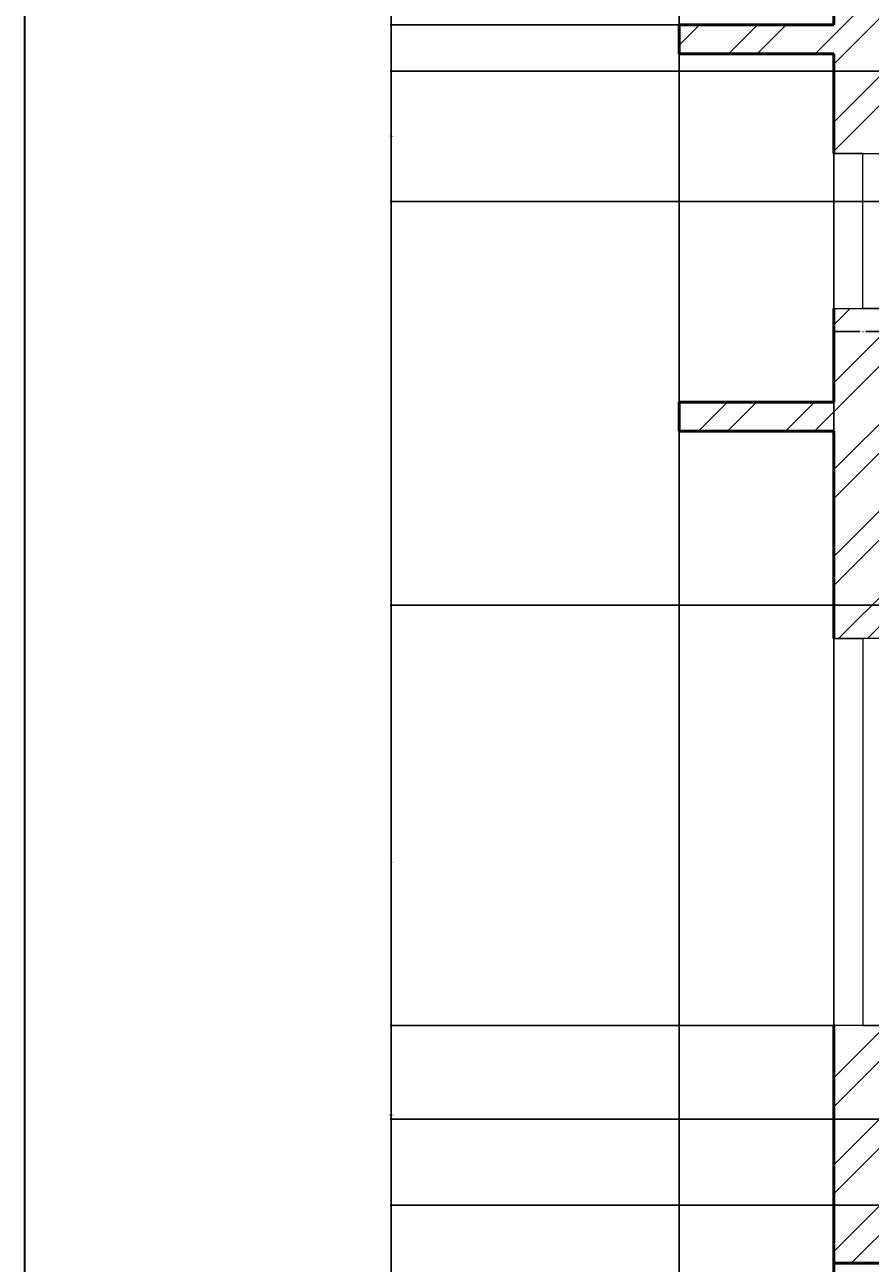
# Model space of a CAD drawing. Units: inches. Extents: x 1980 to 2738, y 1471 to 2568.
# Tile 2 of 22: x 1980 to 2111, y 1686 to 1878. Entities that reach past the tile are written whole.
import ezdxf

# ---------------------------------------------------------------- set-up
doc = ezdxf.new("R2010")
doc.units = ezdxf.units.IN
for name, color, linetype, lineweight in [('A-ANNO-DIMS', 2, 'Continuous', 18), ('A-ANNO-TTLB', 7, 'Continuous', 35), ('A-FLOR-BALC', 7, 'Continuous', 25), ('A-GLAZ', 141, 'Continuous', 18), ('A-WALL', 7, 'Continuous', 50)]:
    doc.layers.add(name, color=color, linetype=linetype, lineweight=lineweight)
doc.layers.add('A-WALL-PATT', color=9, linetype='Continuous', lineweight=13, true_color=0xd19cc7)
doc.styles.get("Standard").update_dxf_attribs({"font": 'arial.ttf'})
doc.dimstyles.get("Standard").update_dxf_attribs({"dimtxt": 0.18, "dimasz": 0.18, "dimexe": 0.18, "dimexo": 0.0625, "dimgap": 0.09, "dimtad": 0, "dimtih": 1, "dimtoh": 1, "dimdec": 4, "dimzin": 0, "dimdsep": 46, "dimtxsty": 'Standard', "dimcen": 0.09, "dimadec": 0, "dimazin": 0, "dimtfac": 1, "dimtdec": 4, "dimtofl": 0, "dimtmove": 0, "dimatfit": 3, "dimfxl": 1, "dimtolj": 1, "dimtzin": 0, "dimarcsym": 0})

# ---------------------------------------------------------------- blocks, each defined once
blk = doc.blocks.new('WIN-60IN-WALL')
for p, q in [((0, 9), (0, 0)), ((60, 9), (0, 9)), ((60, 4.5), (60, 9)), ((60, 9), (60, 0)), ((0, 0), (0, 4.5)), ((0, 4.5), (60, 4.5)), ((0, 0), (60, 0))]:
    blk.add_line(p, q)
blk = doc.blocks.new('WIN-24IN-WALL')
for p, q in [((4.5, 24), (0, 24)), ((0, 24), (9, 24)), ((0, 24), (0, 0)), ((4.5, 0), (4.5, 24)), ((9, 0), (9, 24)), ((0, 0), (9, 0)), ((9, 0), (4.5, 0))]:
    blk.add_line(p, q)
blk = doc.blocks.new('*D24')
at = {"layer": 'A-ANNO-DIMS', "color": 0, "lineweight": -2, "transparency": 16777216}
for p, q in [((2105.08, 1833.67), (2105.08, 1829.95)), ((2114.08, 1833.67), (2114.08, 1829.95)), ((2105.26, 1830.13), (2109.13, 1830.13)), ((2113.9, 1830.13), (2110.04, 1830.13))]:
    blk.add_line(p, q, dxfattribs=at)
at = {"layer": 'A-ANNO-DIMS', "color": 0, "transparency": 16777216}
for points in [[(2105.26, 1830.16), (2105.26, 1830.1), (2105.08, 1830.13)], [(2113.9, 1830.16), (2113.9, 1830.1), (2114.08, 1830.13)]]:
    blk.add_solid(points, dxfattribs=at)
at = {"layer": 'Defpoints', "color": 0, "transparency": 16777216}
for p in [(2105.08, 1833.73), (2114.08, 1833.73), (2114.08, 1830.13)]:
    blk.add_point(p, dxfattribs=at)
at = {"layer": 'A-ANNO-DIMS', "color": 0, "transparency": 16777216, "insert": (2109.58, 1830.13), "char_height": 0.18, "attachment_point": 5}
blk.add_mtext('\\A1;9 TYP.', dxfattribs=at)
blk = doc.blocks.new('*D36')
at = {"layer": 'A-ANNO-DIMS', "color": 0, "lineweight": -2, "transparency": 16777216}
for p, q in [((2105.02, 2462.71), (2036.25, 2462.71)), ((2036.43, 2462.53), (2036.43, 2053.39)), ((2036.43, 1643.89), (2036.43, 2053.02)), ((2105.02, 1643.71), (2036.25, 1643.71))]:
    blk.add_line(p, q, dxfattribs=at)
at = {"layer": 'A-ANNO-DIMS', "color": 0, "transparency": 16777216}
for points in [[(2036.4, 2462.53), (2036.46, 2462.53), (2036.43, 2462.71)], [(2036.4, 1643.89), (2036.46, 1643.89), (2036.43, 1643.71)]]:
    blk.add_solid(points, dxfattribs=at)
at = {"layer": 'Defpoints', "color": 0, "transparency": 16777216}
for p in [(2036.43, 2462.71), (2105.08, 2462.71), (2105.08, 1643.71)]:
    blk.add_point(p, dxfattribs=at)
at = {"layer": 'A-ANNO-DIMS', "color": 0, "transparency": 16777216, "insert": (2036.43, 2053.21), "char_height": 0.18, "attachment_point": 5}
blk.add_mtext('\\A1;819', dxfattribs=at)
blk = doc.blocks.new('*D48')
at = {"layer": 'A-ANNO-DIMS', "color": 0, "lineweight": -2, "transparency": 16777216}
for p, q in [((2081.08, 1873.14), (2081.08, 1533.71)), ((2105.08, 1873.14), (2105.08, 1533.71)), ((2081.26, 1533.89), (2092.86, 1533.89)), ((2104.9, 1533.89), (2093.3, 1533.89))]:
    blk.add_line(p, q, dxfattribs=at)
at = {"layer": 'A-ANNO-DIMS', "color": 0, "transparency": 16777216}
for points in [[(2081.26, 1533.92), (2081.26, 1533.86), (2081.08, 1533.89)], [(2104.9, 1533.92), (2104.9, 1533.86), (2105.08, 1533.89)]]:
    blk.add_solid(points, dxfattribs=at)
at = {"layer": 'Defpoints', "color": 0, "transparency": 16777216}
for p in [(2081.08, 1873.21), (2105.08, 1873.21), (2105.08, 1533.89)]:
    blk.add_point(p, dxfattribs=at)
at = {"layer": 'A-ANNO-DIMS', "color": 0, "transparency": 16777216, "insert": (2093.08, 1533.89), "char_height": 0.18, "attachment_point": 5}
blk.add_mtext('\\A1;24', dxfattribs=at)
blk = doc.blocks.new('*D49')
at = {"layer": 'A-ANNO-DIMS', "color": 0, "lineweight": -2, "transparency": 16777216}
for p, q in [((2105.02, 1722.55), (2036.25, 1722.55)), ((2036.43, 1722.37), (2036.43, 1708.81)), ((2036.43, 1694.89), (2036.43, 1708.45)), ((2114.02, 1694.71), (2036.25, 1694.71))]:
    blk.add_line(p, q, dxfattribs=at)
at = {"layer": 'A-ANNO-DIMS', "color": 0, "transparency": 16777216}
for points in [[(2036.4, 1722.37), (2036.46, 1722.37), (2036.43, 1722.55)], [(2036.4, 1694.89), (2036.46, 1694.89), (2036.43, 1694.71)]]:
    blk.add_solid(points, dxfattribs=at)
at = {"layer": 'Defpoints', "color": 0, "transparency": 16777216}
for p in [(2036.43, 1722.55), (2105.08, 1722.55), (2114.08, 1694.71)]:
    blk.add_point(p, dxfattribs=at)
at = {"layer": 'A-ANNO-DIMS', "color": 0, "transparency": 16777216, "insert": (2036.43, 1708.63), "char_height": 0.18, "attachment_point": 5}
blk.add_mtext('\\A1;27.845', dxfattribs=at)
blk = doc.blocks.new('*D52')
at = {"layer": 'A-ANNO-DIMS', "color": 0, "lineweight": -2, "transparency": 16777216}
for p, q in [((2341.71, 1787.71), (2036.25, 1787.71)), ((2036.43, 1787.53), (2036.43, 1748.05)), ((2036.43, 1708.21), (2036.43, 1747.69)), ((2341.71, 1708.03), (2036.25, 1708.03))]:
    blk.add_line(p, q, dxfattribs=at)
at = {"layer": 'A-ANNO-DIMS', "color": 0, "transparency": 16777216}
for points in [[(2036.4, 1787.53), (2036.46, 1787.53), (2036.43, 1787.71)], [(2036.4, 1708.21), (2036.46, 1708.21), (2036.43, 1708.03)]]:
    blk.add_solid(points, dxfattribs=at)
at = {"layer": 'Defpoints', "color": 0, "transparency": 16777216}
for p in [(2036.43, 1787.71), (2341.78, 1787.71), (2341.78, 1708.03)]:
    blk.add_point(p, dxfattribs=at)
at = {"layer": 'A-ANNO-DIMS', "color": 0, "transparency": 16777216, "insert": (2036.43, 1747.87), "char_height": 0.18, "attachment_point": 5}
blk.add_mtext('\\A1;79.68', dxfattribs=at)
blk = doc.blocks.new('*D62')
at = {"layer": 'A-ANNO-DIMS', "color": 0, "lineweight": -2, "transparency": 16777216}
for p, q in [((2105.02, 1890.1), (2036.25, 1890.1)), ((2036.43, 1889.92), (2036.43, 1884.08)), ((2036.43, 1877.89), (2036.43, 1883.72)), ((2105.02, 1877.71), (2036.25, 1877.71))]:
    blk.add_line(p, q, dxfattribs=at)
at = {"layer": 'A-ANNO-DIMS', "color": 0, "transparency": 16777216}
for points in [[(2036.4, 1889.92), (2036.46, 1889.92), (2036.43, 1890.1)], [(2036.4, 1877.89), (2036.46, 1877.89), (2036.43, 1877.71)]]:
    blk.add_solid(points, dxfattribs=at)
at = {"layer": 'Defpoints', "color": 0, "transparency": 16777216}
for p in [(2036.43, 1890.1), (2105.08, 1890.1), (2105.08, 1877.71)]:
    blk.add_point(p, dxfattribs=at)
at = {"layer": 'A-ANNO-DIMS', "color": 0, "transparency": 16777216, "insert": (2036.43, 1883.9), "char_height": 0.18, "attachment_point": 5}
blk.add_mtext('\\A1;12.39', dxfattribs=at)
blk = doc.blocks.new('*D65')
at = {"layer": 'A-ANNO-DIMS', "color": 0, "lineweight": -2, "transparency": 16777216}
for p, q in [((2293.25, 1870.5), (2036.25, 1870.5)), ((2036.43, 1870.32), (2036.43, 1860.58)), ((2036.43, 1850.47), (2036.43, 1860.21)), ((2293.25, 1850.29), (2036.25, 1850.29))]:
    blk.add_line(p, q, dxfattribs=at)
at = {"layer": 'A-ANNO-DIMS', "color": 0, "transparency": 16777216}
for points in [[(2036.4, 1870.32), (2036.46, 1870.32), (2036.43, 1870.5)], [(2036.4, 1850.47), (2036.46, 1850.47), (2036.43, 1850.29)]]:
    blk.add_solid(points, dxfattribs=at)
at = {"layer": 'Defpoints', "color": 0, "transparency": 16777216}
for p in [(2036.43, 1870.5), (2293.31, 1870.5), (2293.31, 1850.29)]:
    blk.add_point(p, dxfattribs=at)
at = {"layer": 'A-ANNO-DIMS', "color": 0, "transparency": 16777216, "insert": (2036.43, 1860.4), "char_height": 0.18, "attachment_point": 5}
blk.add_mtext('\\A1;20.204', dxfattribs=at)

msp = doc.modelspace()

# ---------------------------------------------------------------- hatches: boundary and pattern name
at = {"layer": 'A-WALL-PATT'}
h = msp.add_hatch(dxfattribs=at)
h.set_pattern_fill('ANSI32', color=256)
h.paths.add_polyline_path([(2257.5661, 2416.2064), (2257.5661, 2420.7064), (2250.5833, 2420.7064), (2250.5833, 2462.7064), (2246.0833, 2462.7064), (2246.0833, 2420.7064), (2237.0791, 2420.7064), (2237.0791, 2411.7064), (2246.0833, 2411.7064), (2246.0833, 2291.7064), (2242.6109, 2291.7064), (2242.6109, 2287.2064), (2246.0833, 2287.2064), (2250.5833, 2287.2064), (2250.5833, 2291.7064), (2250.5833, 2411.7064), (2257.5661, 2411.7064)])
h.paths.add_polyline_path([(2387.0396, 2416.2064), (2387.0396, 2420.7064), (2367.5833, 2420.7064), (2367.5833, 2462.7064), (2358.5833, 2462.7064), (2358.5833, 2420.7064), (2329.3087, 2420.7064), (2329.3087, 2411.7064), (2358.5833, 2411.7064), (2358.5833, 2321.7275), (2358.5833, 2309.7064), (2347.3089, 2309.7064), (2293.3089, 2309.7064), (2293.3089, 2259.0771), (2297.8089, 2259.0771), (2297.8089, 2305.2064), (2347.3089, 2305.2064), (2347.3089, 2284.7412), (2351.8089, 2284.7412), (2351.8089, 2305.2064), (2372.3188, 2305.2064), (2372.3761, 2284.3899), (2377.0295, 2284.3899), (2377.0295, 2299.3058), (2377.0295, 2305.2064), (2426.5295, 2305.2064), (2426.5295, 2257.5573), (2431.0295, 2257.5573), (2431.0295, 2309.7064), (2377.0295, 2309.7064), (2367.5833, 2309.7064), (2367.5833, 2321.7275), (2367.5833, 2411.7064), (2387.0396, 2411.7064)])
h.paths.add_polyline_path([(2448.5267, 2416.2064), (2448.5267, 2420.7064), (2423.0396, 2420.7064), (2423.0396, 2411.7064), (2448.5267, 2411.7064)])
h.paths.add_polyline_path([(2130.9128, 2416.2064), (2130.9128, 2420.7064), (2105.0833, 2420.7064), (2105.0833, 2386.6942), (2114.0833, 2386.6942), (2114.0833, 2411.7064), (2130.9128, 2411.7064)])
h.paths.add_polyline_path([(2212.9478, 2420.7064), (2190.9128, 2420.7064), (2190.9128, 2411.7064), (2212.9478, 2411.7064), (2212.9478, 2416.2064)])
h.paths.add_polyline_path([(2114.0833, 2326.6942), (2105.0833, 2326.6942), (2105.0833, 2291.7064), (2081.0833, 2291.7064), (2081.0833, 2287.2064), (2105.0833, 2287.2064), (2105.0833, 2276.1935), (2114.0833, 2276.1935), (2114.0833, 2287.2064), (2166.3825, 2287.2064), (2166.3825, 2289.4564), (2166.3825, 2291.7064), (2114.0833, 2291.7064)])
h.paths.add_polyline_path([(2114.0833, 2252.1935), (2105.0833, 2252.1935), (2105.0833, 2233.2064), (2081.0833, 2233.2064), (2081.0833, 2228.7064), (2105.0833, 2228.7064), (2105.0833, 2213.4478), (2114.0833, 2213.4478), (2114.0833, 2228.7064), (2195.0833, 2228.7064), (2199.5833, 2228.7064), (2208.4455, 2228.7064), (2208.4455, 2230.9564), (2208.4455, 2233.2064), (2199.5833, 2233.2064), (2199.5833, 2287.2064), (2206.8904, 2287.2064), (2206.8904, 2289.4564), (2206.8904, 2291.7064), (2189.446, 2291.7064), (2189.446, 2289.4564), (2189.446, 2287.2064), (2195.0833, 2287.2064), (2195.0833, 2233.2064), (2114.0833, 2233.2064)])
h.paths.add_polyline_path([(2114.0833, 2153.4478), (2109.5833, 2153.4478), (2105.0833, 2153.4478), (2105.0833, 2135.2374), (2114.0833, 2135.2374)], flags=17)
h.paths.add_polyline_path([(2135.9619, 2095.4081), (2140.1805, 2095.4081), (2140.1805, 2104.2064), (2114.0833, 2104.2064), (2114.0833, 2110.3997), (2109.5833, 2110.3997), (2105.0833, 2110.3997), (2105.0833, 2104.2064), (2081.0833, 2104.2064), (2081.0833, 2099.7064), (2105.0833, 2099.7064), (2127.5416, 2099.8532), (2127.5416, 2056.9393), (2136.2133, 2056.9393)], flags=17)
h.paths.add_polyline_path([(2255.4895, 2104.2064), (2250.5833, 2104.2064), (2250.5833, 2233.2064), (2246.0833, 2233.2064), (2242.4941, 2233.2064), (2242.4941, 2228.7064), (2246.0833, 2228.7064), (2246.0833, 2104.2064), (2163.6825, 2104.2064), (2163.6825, 2099.8072), (2163.6825, 2095.4081), (2191.4325, 2095.4081), (2191.4325, 2011.2064), (2186.0833, 2011.2064), (2136.5143, 2010.8824), (2136.3702, 2032.9403), (2131.9559, 2032.9115), (2127.5416, 2032.8826), (2127.5416, 2006.7064), (2105.0833, 2006.7064), (2081.0833, 2006.7064), (2081.0833, 2002.2064), (2105.0833, 2002.2064), (2105.0833, 1995.9329), (2114.0833, 1995.9329), (2114.0833, 2002.2064), (2246.0833, 2002.2064), (2246.0833, 1877.7064), (2242.1358, 1877.7064), (2242.1358, 1873.2064), (2250.5833, 1873.2064), (2250.5833, 2002.2064), (2255.3335, 2002.2064), (2255.3335, 2011.2064), (2195.9325, 2011.2064), (2195.9325, 2095.2064), (2255.4895, 2095.2064), (2255.4895, 2099.5471)])
h.paths.add_polyline_path([(2199.5833, 1873.2064), (2209.827, 1873.2064), (2209.827, 1875.4564), (2209.827, 1877.7064), (2114.0833, 1877.7064), (2114.0833, 1890.0968), (2105.0833, 1890.0968), (2105.0833, 1877.7064), (2081.0833, 1877.7064), (2081.0833, 1873.2064), (2105.0833, 1873.2064), (2105.0833, 1857.7279), (2114.0833, 1857.7279), (2114.0833, 1873.2064), (2195.0833, 1873.2064), (2195.0833, 1819.2064), (2190.298, 1819.2064), (2190.298, 1814.7064), (2209.8976, 1814.7064), (2209.8976, 1816.9564), (2209.8976, 1819.2064), (2199.5833, 1819.2064)])
h.paths.add_polyline_path([(2114.0833, 1814.7064), (2166.2538, 1814.7064), (2166.2538, 1816.9564), (2166.2538, 1819.2064), (2114.0833, 1819.2064), (2114.0833, 1833.7279), (2109.5833, 1833.7279), (2105.0833, 1833.7279), (2105.0833, 1819.2064), (2081.0833, 1819.2064), (2081.0833, 1814.7064), (2105.0833, 1814.7064), (2105.0833, 1782.5516), (2114.0833, 1782.5516)])
h.paths.add_polyline_path([(2114.0833, 1722.5516), (2109.5833, 1722.5516), (2105.0833, 1722.5516), (2105.0833, 1685.7064), (2124.5104, 1685.7064), (2124.5104, 1690.2064), (2124.5104, 1694.7064), (2114.0833, 1694.7064)])
h.paths.add_polyline_path([(2218.8787, 1694.7064), (2184.5104, 1694.7064), (2184.5104, 1685.7064), (2218.8787, 1685.7064), (2218.8787, 1690.2064)])
h.paths.add_polyline_path([(2250.5833, 1819.2064), (2242.6431, 1819.2064), (2242.6431, 1816.9564), (2242.6431, 1814.7064), (2246.0833, 1814.7064), (2246.0833, 1694.7064), (2240.4035, 1694.7064), (2240.4035, 1690.2064), (2240.4035, 1685.7064), (2246.0833, 1685.7064), (2246.0833, 1643.7064), (2250.5833, 1643.7064), (2250.5833, 1685.7064), (2255.9859, 1685.7064), (2255.9859, 1690.2064), (2255.9859, 1694.7064), (2250.5833, 1694.7064)])
h.paths.add_polyline_path([(2297.4764, 1694.7064), (2279.3934, 1694.7064), (2279.3934, 1690.2064), (2279.3934, 1685.7064), (2297.4764, 1685.7064), (2297.4764, 1690.2064)])
h.paths.add_polyline_path([(2377.1596, 1694.7064), (2367.5833, 1694.7064), (2367.5833, 1787.7064), (2431.0295, 1787.7064), (2431.0295, 1792.2064), (2431.0295, 1849.4149), (2428.7795, 1849.4149), (2426.5295, 1849.4149), (2426.5295, 1792.2064), (2421.5833, 1792.2064), (2367.5833, 1792.2064), (2297.8089, 1792.2064), (2297.8089, 1850.2946), (2295.5589, 1850.2946), (2293.3089, 1850.2946), (2293.3089, 1792.2064), (2293.3089, 1787.7064), (2297.8089, 1787.7064), (2358.5833, 1787.7064), (2358.5833, 1694.7064), (2333.4764, 1694.7064), (2333.4764, 1685.7064), (2358.5833, 1685.7064), (2358.5833, 1643.7064), (2367.5833, 1643.7064), (2367.5833, 1685.7064), (2377.1596, 1685.7064)])
h.paths.add_polyline_path([(2442.4912, 1694.7064), (2413.1596, 1694.7064), (2413.1596, 1685.7064), (2442.4912, 1685.7064)])
h.paths.add_polyline_path([(2480.0833, 1814.7064), (2483.4816, 1814.7064), (2483.4816, 1817.9384), (2483.4816, 1819.2064), (2475.5833, 1819.2064), (2475.5833, 1694.7064), (2470.7283, 1694.7064), (2470.7283, 1685.7064), (2475.5833, 1685.7064), (2475.5833, 1643.7064), (2480.0833, 1643.7064), (2480.0833, 1685.7064), (2486.3293, 1685.7064), (2486.3293, 1690.2064), (2486.3293, 1694.7064), (2480.0833, 1694.7064)])
h.paths.add_polyline_path([(2621.0833, 1721.7349), (2612.0833, 1721.7349), (2612.0833, 1694.7064), (2586.1453, 1694.7064), (2586.1453, 1685.7064), (2621.0833, 1685.7064)])
h.paths.add_polyline_path([(2526.1453, 1690.2064), (2526.1453, 1694.7064), (2511.584, 1694.7064), (2511.584, 1690.2064), (2511.584, 1685.7064), (2526.1453, 1685.7064)])
h.paths.add_polyline_path([(2645.0833, 1819.2064), (2621.0833, 1819.2064), (2621.0833, 1835.8527), (2616.5833, 1835.8527), (2612.0833, 1835.8527), (2612.0833, 1819.2064), (2560.2541, 1819.2064), (2560.2541, 1814.7064), (2612.0833, 1814.7064), (2612.0833, 1781.7349), (2621.0833, 1781.7349), (2621.0833, 1814.7064), (2645.0833, 1814.7064)])
h.paths.add_polyline_path([(2645.0833, 1877.7064), (2621.0833, 1877.7064), (2621.0833, 1886.4375), (2612.0833, 1886.4375), (2612.0833, 1877.7064), (2517.1032, 1877.7064), (2517.1032, 1875.4564), (2517.1032, 1873.2064), (2526.5833, 1873.2064), (2526.5833, 1819.2064), (2516.6454, 1819.2064), (2516.6454, 1816.9564), (2516.6454, 1814.7064), (2536.4445, 1814.7064), (2536.4445, 1816.9564), (2536.4445, 1819.2064), (2531.0833, 1819.2064), (2531.0833, 1873.2064), (2612.0833, 1873.2064), (2612.0833, 1859.8527), (2621.0833, 1859.8527), (2621.0833, 1873.2064), (2645.0833, 1873.2064)])
h.paths.add_polyline_path([(2645.0833, 2006.7064), (2621.0833, 2006.7064), (2588.5085, 2006.7064), (2588.5085, 2052.9125), (2579.9045, 2052.9125), (2579.9045, 2011.2064), (2519.9045, 2011.2064), (2519.9045, 2095.2064), (2553.1204, 2095.2064), (2553.1204, 2104.2064), (2480.0833, 2104.2064), (2480.0833, 2228.7064), (2484.3832, 2228.7064), (2484.3832, 2230.9564), (2484.3832, 2233.2064), (2475.5833, 2233.2064), (2475.5833, 2104.2064), (2463.1308, 2104.2064), (2463.1308, 2095.2064), (2501.2463, 2095.2064), (2510.9045, 2095.2064), (2515.4045, 2095.2064), (2515.4045, 2011.2064), (2510.9045, 2011.2064), (2501.2463, 2011.2064), (2462.5957, 2011.2064), (2462.5957, 2002.2064), (2475.5833, 2002.2064), (2475.5833, 1873.2064), (2483.6146, 1873.2064), (2483.6146, 1875.4564), (2483.6146, 1877.7064), (2480.0833, 1877.7064), (2480.0833, 2002.2064), (2612.0833, 2002.2064), (2612.0833, 1996.309), (2621.0833, 1996.309), (2621.0833, 2002.2064), (2645.0833, 2002.2064)])
h.paths.add_polyline_path([(2588.5085, 2099.7277), (2621.0833, 2099.7277), (2645.0833, 2099.7064), (2645.0833, 2104.2064), (2621.0833, 2104.2064), (2621.0833, 2109.0038), (2616.5833, 2109.0038), (2612.0833, 2109.0038), (2612.0833, 2104.2064), (2575.0621, 2104.2064), (2575.0621, 2099.7064), (2575.0621, 2095.2064), (2579.9045, 2095.2064), (2579.9045, 2076.9125), (2588.5085, 2076.9125)], flags=17)
h.paths.add_polyline_path([(2367.5833, 2002.2064), (2373.7228, 2002.2064), (2373.7228, 2006.7064), (2373.7228, 2011.2064), (2350.7889, 2011.2064), (2350.7889, 2006.7064), (2350.7889, 2002.2064), (2358.5833, 2002.2064), (2358.5833, 1877.7064), (2293.3089, 1877.7064), (2293.3089, 1870.4987), (2297.8089, 1870.4987), (2297.8089, 1873.2064), (2347.3089, 1873.2064), (2347.3089, 1847.2208), (2351.8089, 1847.2208), (2351.8089, 1873.2064), (2372.5295, 1873.2064), (2372.5295, 1847.8619), (2377.0295, 1847.8619), (2377.0295, 1873.2064), (2426.5295, 1873.2064), (2426.5295, 1868.7339), (2431.0295, 1868.7339), (2431.0295, 1877.7064), (2367.5833, 1877.7064)])
h.paths.add_polyline_path([(2531.0833, 2287.2064), (2534.2285, 2287.2064), (2534.2285, 2291.7064), (2516.7886, 2291.7064), (2516.7886, 2287.2064), (2526.5833, 2287.2064), (2526.5833, 2233.2064), (2517.9112, 2233.2064), (2517.9112, 2230.9564), (2517.9112, 2228.7064), (2526.5833, 2228.7064), (2531.0833, 2228.7064), (2612.0833, 2228.7064), (2612.0833, 2206.8504), (2621.0833, 2206.8504), (2621.0833, 2228.7064), (2645.0833, 2228.7064), (2645.0833, 2233.2064), (2621.0833, 2233.2064), (2621.0833, 2241.8536), (2616.5833, 2241.8536), (2612.0833, 2241.8536), (2612.0833, 2233.2064), (2531.0833, 2233.2064)])
h.paths.add_polyline_path([(2645.0833, 2291.7064), (2621.0833, 2291.7064), (2621.0833, 2323.0138), (2616.5833, 2323.0138), (2612.0833, 2323.0138), (2612.0833, 2291.7064), (2559.6852, 2291.7064), (2559.6852, 2289.4564), (2559.6852, 2287.2064), (2612.0833, 2287.2064), (2612.0833, 2265.8536), (2621.0833, 2265.8536), (2621.0833, 2287.2064), (2645.0833, 2287.2064)])
h.paths.add_polyline_path([(2621.0833, 2420.7064), (2582.8189, 2420.7064), (2582.8189, 2411.7064), (2612.0833, 2411.7064), (2612.0833, 2383.0138), (2621.0833, 2383.0138)])
h.paths.add_polyline_path([(2480.0833, 2411.7064), (2485.7342, 2411.7064), (2485.7342, 2416.2064), (2485.7342, 2420.7064), (2480.0833, 2420.7064), (2480.0833, 2462.7064), (2475.5833, 2462.7064), (2475.5833, 2420.7064), (2469.4083, 2420.7064), (2469.4083, 2411.7064), (2475.5833, 2411.7064), (2475.5833, 2291.7064), (2475.5833, 2287.2064), (2482.9195, 2287.2064), (2482.9195, 2289.4564), (2482.9195, 2291.7064), (2480.0833, 2291.7064)])
h.paths.add_polyline_path([(2367.5833, 2228.7064), (2431.0295, 2228.7064), (2431.0295, 2233.2064), (2431.0295, 2237.4203), (2428.7795, 2237.4203), (2426.5295, 2237.4203), (2426.5295, 2233.2064), (2377.0295, 2233.2064), (2377.0295, 2260.3837), (2372.4423, 2260.3837), (2372.517, 2233.2635), (2351.8089, 2233.2064), (2351.8089, 2260.7412), (2347.3089, 2260.7412), (2347.3089, 2233.2064), (2297.8089, 2233.2064), (2297.8089, 2236.9324), (2293.3089, 2236.9324), (2293.3089, 2228.7064), (2358.5833, 2228.7064), (2358.5833, 2104.2064), (2353.3665, 2104.2064), (2353.3665, 2095.2064), (2373.8869, 2095.2064), (2373.8869, 2099.7064), (2373.8869, 2104.2064), (2367.5833, 2104.2064)])
h.paths.add_polyline_path([(2321.2323, 2104.2064), (2303.4895, 2104.2064), (2303.4895, 2095.2064), (2321.2323, 2095.2064), (2321.2323, 2099.7064)], flags=0)
h.paths.add_polyline_path([(2415.1308, 2099.7064), (2415.1308, 2104.2064), (2404.81, 2104.2064), (2404.81, 2095.2064), (2415.1308, 2095.2064)], flags=17)
h.paths.add_polyline_path([(2318.6336, 2011.2064), (2303.3335, 2011.2064), (2303.3335, 2002.2064), (2318.6336, 2002.2064)], flags=0)
h.paths.add_polyline_path([(2414.5957, 2011.2064), (2406.2461, 2011.2064), (2406.2461, 2006.7064), (2406.2461, 2002.2064), (2414.5957, 2002.2064)], flags=17)

# ---------------------------------------------------------------- linework, layer by layer
at = {"layer": 'A-ANNO-TTLB'}
msp.add_lwpolyline([(1979.5621, 2567.5568), (2738.2543, 2567.5568), (2738.2543, 1471.317), (1979.5621, 1471.317)], close=True, dxfattribs=at)
at = {"layer": 'A-FLOR-BALC'}
msp.add_line((2081.0833, 2287.2064), (2081.0833, 1819.2064), dxfattribs=at)
at = {"layer": 'A-WALL'}
for p, q in [((2105.0833, 1902.4872), (2105.0833, 1877.7064)), ((2105.0833, 1877.7064), (2081.0833, 1877.7064)), ((2081.0833, 1877.7064), (2081.0833, 1873.2064)), ((2081.0833, 1873.2064), (2105.0833, 1873.2064)), ((2105.0833, 1873.2064), (2105.0833, 1857.7279)), ((2105.0833, 1833.7279), (2105.0833, 1819.2064)), ((2105.0833, 1819.2064), (2081.0833, 1819.2064)), ((2081.0833, 1819.2064), (2081.0833, 1814.7064)), ((2081.0833, 1814.7064), (2105.0833, 1814.7064)), ((2105.0833, 1814.7064), (2105.0833, 1782.5516)), ((2105.0833, 1722.5516), (2105.0833, 1643.7064)), ((2124.5104, 1685.7064), (2105.0833, 1685.7064))]:
    msp.add_line(p, q, dxfattribs=at)

# ---------------------------------------------------------------- block references
at = {"layer": 'A-GLAZ'}
msp.add_blockref('WIN-24IN-WALL', (2105.083, 1833.7283), dxfattribs=at)
at = {"layer": 'A-GLAZ', "rotation": 270}
msp.add_blockref('WIN-60IN-WALL', (2105.0828, 1782.5514), dxfattribs=at)

# ---------------------------------------------------------------- dimensions: what is measured, and where the dimension line sits
at = {"layer": 'A-ANNO-DIMS'}
for base, p1, p2, override, picture, middle in [((2036.4333, 2462.7064), (2105.0833, 1643.7064), (2105.0833, 2462.7064), {"dimdec": 0, "dimlfac": 1, "dimrnd": 0, "dimzin": 0, "dimdsep": 46, "dimlunit": 2}, '*D36', (2036.4333, 2053.2064)), ((2036.4333, 1890.0968), (2105.0833, 1877.7064), (2105.0833, 1890.0968), {"dimdec": 2, "dimlfac": 1, "dimrnd": 0, "dimzin": 0, "dimdsep": 46, "dimlunit": 2}, '*D62', (2036.4333, 1883.9016)), ((2036.4333, 1870.4987), (2293.3089, 1850.2946), (2293.3089, 1870.4987), {"dimdec": 3, "dimlfac": 1, "dimrnd": 0, "dimzin": 0, "dimdsep": 46, "dimlunit": 2}, '*D65', (2036.4333, 1860.3966)), ((2036.4333, 1787.7064), (2341.776, 1708.0291), (2341.776, 1787.7064), {"dimdec": 2, "dimlfac": 1, "dimrnd": 0, "dimzin": 0, "dimdsep": 46, "dimlunit": 2}, '*D52', (2036.4333, 1747.8678)), ((2036.4333, 1722.5516), (2114.0833, 1694.7064), (2105.0833, 1722.5516), {"dimdec": 3, "dimlfac": 1, "dimrnd": 0, "dimzin": 0, "dimdsep": 46, "dimlunit": 2}, '*D49', (2036.4333, 1708.629))]:
    dim = msp.add_linear_dim(base=base, p1=p1, p2=p2, angle=90, dimstyle='Standard', override=override, dxfattribs=at)
    dim.commit()
    dim.dimension.update_dxf_attribs({"geometry": picture, "text_midpoint": middle})
dim = msp.add_linear_dim(base=(2105.0833, 1533.8857), p1=(2081.0833, 1873.2064), p2=(2105.0833, 1873.2064), dimstyle='Standard', override={"dimdec": 0, "dimlfac": 1, "dimrnd": 0, "dimzin": 0, "dimdsep": 46, "dimlunit": 2}, dxfattribs=at)
dim.commit()
dim.dimension.update_dxf_attribs({"geometry": '*D48', "text_midpoint": (2093.0833, 1533.8857)})
dim = msp.add_linear_dim(base=(2114.0833, 1830.1279), p1=(2105.0833, 1833.7279), p2=(2114.0833, 1833.7279), text='<> TYP.', dimstyle='Standard', override={"dimdec": 0, "dimlfac": 1, "dimrnd": 0, "dimzin": 0, "dimdsep": 46, "dimlunit": 2}, dxfattribs=at)
dim.commit()
dim.dimension.update_dxf_attribs({"geometry": '*D24', "text_midpoint": (2109.5833, 1830.1279)})

doc.saveas('drawing.dxf')
